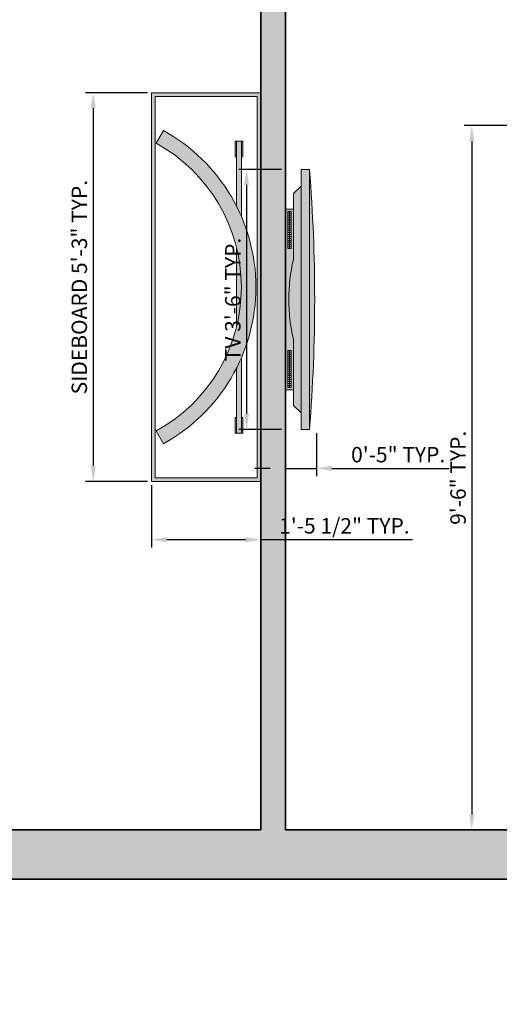
# Model space of a CAD drawing. Units: inches. Extents: x 1566 to 2546, y 1087 to 2705.
# Tile 14 of 27: x 2237 to 2315, y 1189 to 1349. Entities that reach past the tile are written whole.
import ezdxf

# ---------------------------------------------------------------- set-up
doc = ezdxf.new("R2010")
doc.units = ezdxf.units.IN
for name, color, linetype, lineweight in [('A-ANNO-DIMS', 2, 'Continuous', 18), ('A-FURN', 8, 'Continuous', 18), ('A-WALL', 7, 'Continuous', 35), ('A-WALL-PATT', 8, 'Continuous', 13), ('aparador', 36, 'Continuous', 9), ('moveis', 254, 'Continuous', 5), ('parede', 7, 'Continuous', 30)]:
    doc.layers.add(name, color=color, linetype=linetype, lineweight=lineweight)
doc.styles.get("Standard").update_dxf_attribs({"font": 'arial.ttf'})
doc.dimstyles.new('ISO-25', dxfattribs={"dimtxt": 2.5, "dimasz": 2.5, "dimexe": 1.25, "dimexo": 0.625, "dimtad": 1, "dimtxsty": 'Standard', "dimcen": 2.5, "dimadec": 0, "dimazin": 0, "dimtfac": 1, "dimtmove": 0, "dimatfit": 3, "dimfxl": 1, "dimarcsym": 0})

# ---------------------------------------------------------------- blocks, each defined once
blk = doc.blocks.new('Aparador ORGANICA Formatto')
at = {"layer": 'aparador', "ltscale": 0.3}
h = blk.add_hatch(color=256, dxfattribs=at)
h.dxf.hatch_style = 1
h.set_gradient(color1=(118, 213, 123), color2=(52, 168, 57), one_color=1, tint=0.43, name='INVCURVED')
h.paths.add_polyline_path([(0.8, 0.45), (-0.8, 0.45), (-0.8, 0), (0.8, 0)])
h.paths.add_polyline_path([(0.785, 0.435), (0.785, 0.015), (-0.785, 0.015), (-0.785, 0.435)], flags=16)
h.paths.add_polyline_path([(0.2911, 0.3699), (0.5365, 0.3699), (0.5365, 0.3757), (0.6011, 0.3757), (0.6011, 0.3699), (0.6011, 0.3499), (0.6011, 0.3441), (0.5365, 0.3441), (0.5365, 0.3499), (0.3338, 0.3499, -0.150336), (0.6449, 0.0488), (0.5923, 0.0199, 0.208852), (0.1632, 0.3499), (-0.1632, 0.3499, 0.208852), (-0.5923, 0.0199), (-0.6449, 0.0488, -0.150336), (-0.3338, 0.3499), (-0.5365, 0.3499), (-0.5365, 0.3441), (-0.6011, 0.3441), (-0.6011, 0.3499), (-0.6011, 0.3699), (-0.6011, 0.3757), (-0.5365, 0.3757), (-0.5365, 0.3699), (-0.2911, 0.3699, -0.206106)], flags=0)
h = blk.add_hatch(color=256, dxfattribs=at)
h.dxf.hatch_style = 1
h.set_gradient(color1=(135, 92, 69), color2=(0, 0, 0), one_color=1, name='INVCURVED')
h.paths.add_polyline_path([(-0.6449, 0.0488), (-0.5923, 0.0199, -0.590888), (0.5923, 0.0199), (0.6449, 0.0488, 0.590888)])
h = blk.add_hatch(color=256, dxfattribs=at)
h.dxf.hatch_style = 1
h.set_gradient(color1=(178, 189, 189), one_color=1, tint=1, name='CYLINDER')
h.paths.add_polyline_path([(-0.5365, 0.3757), (-0.6011, 0.3757), (-0.6011, 0.3699), (-0.5365, 0.3699)])
h.paths.add_polyline_path([(-0.5365, 0.3499), (-0.6011, 0.3499), (-0.6011, 0.3441), (-0.5365, 0.3441)])
h = blk.add_hatch(color=256, dxfattribs=at)
h.dxf.hatch_style = 1
h.set_gradient(color1=(118, 213, 123), color2=(31, 101, 35), one_color=1, tint=0.26, name='INVCURVED')
h.paths.add_polyline_path([(-0.2911, 0.3699), (-0.6011, 0.3699), (-0.6011, 0.3499), (-0.3338, 0.3499, -0.015999)])
h = blk.add_hatch(color=256, dxfattribs=at)
h.dxf.hatch_style = 1
h.set_gradient(color1=(118, 213, 123), color2=(31, 101, 35), one_color=1, tint=0.26, name='INVCURVED')
h.paths.add_polyline_path([(-0.1632, 0.3499), (0.1632, 0.3499, 0.122516)])
h = blk.add_hatch(color=256, dxfattribs=at)
h.dxf.hatch_style = 1
h.set_gradient(color1=(118, 213, 123), color2=(31, 101, 35), one_color=1, tint=0.26, name='INVCURVED')
h.paths.add_polyline_path([(0.6011, 0.3699), (0.2911, 0.3699, -0.015999), (0.3338, 0.3499), (0.6011, 0.3499)])
h = blk.add_hatch(color=256, dxfattribs=at)
h.dxf.hatch_style = 1
h.set_gradient(color1=(178, 189, 189), one_color=1, tint=1, name='CYLINDER')
h.paths.add_polyline_path([(0.6011, 0.3757), (0.5365, 0.3757), (0.5365, 0.3699), (0.6011, 0.3699)])
h.paths.add_polyline_path([(0.6011, 0.3499), (0.5365, 0.3499), (0.5365, 0.3441), (0.6011, 0.3441)])
for p, q in [((-0.5923, 0.0199), (-0.6449, 0.0488)), ((0.5923, 0.0199), (0.6449, 0.0488))]:
    blk.add_line(p, q, dxfattribs=at)
for points in [[(-0.6011, 0.3699), (-0.6011, 0.3757), (-0.5365, 0.3757), (-0.5365, 0.3699)], [(0.6011, 0.3699), (0.6011, 0.3757), (0.5365, 0.3757), (0.5365, 0.3699)], [(-0.5365, 0.3499), (-0.5365, 0.3441), (-0.6011, 0.3441), (-0.6011, 0.3499)], [(0.5365, 0.3499), (0.5365, 0.3441), (0.6011, 0.3441), (0.6011, 0.3499)]]:
    blk.add_lwpolyline(points, dxfattribs=at)
for radius in [0.7362, 0.6762]:
    blk.add_arc((0, -0.3063), radius, 28.8434, 151.1566, dxfattribs=at)
at = {"layer": 'moveis', "ltscale": 0.3}
for p, q in [((-0.6011, 0.3699), (-0.6011, 0.3499)), ((-0.2911, 0.3699), (-0.6011, 0.3699)), ((0.2911, 0.3699), (0.6011, 0.3699)), ((0.6011, 0.3699), (0.6011, 0.3499)), ((-0.6011, 0.3499), (-0.3338, 0.3499)), ((-0.1632, 0.3499), (0.1632, 0.3499)), ((0.6011, 0.3499), (0.3338, 0.3499))]:
    blk.add_line(p, q, dxfattribs=at)
for points in [[(-0.8, 0), (0.8, 0), (0.8, 0.45), (-0.8, 0.45)], [(-0.785, 0.015), (0.785, 0.015), (0.785, 0.435), (-0.785, 0.435)]]:
    blk.add_lwpolyline(points, close=True, dxfattribs=at)
blk = doc.blocks.new('PLASMA 2')
at = {"layer": 'moveis', "ltscale": 0.08}
h = blk.add_hatch(dxfattribs=at)
h.set_pattern_fill('_USER,_O', color=256, scale=0.008, double=1, pattern_type=0)
h.set_pattern_definition([(360, (-4.134502, -6.848382), (0, 0.008), []), (90, (-4.134502, -6.848382), (-0.008, 0), [])])
h.paths.add_polyline_path([(-0.2099, -0.0965), (-0.3623, -0.0965), (-0.3623, -0.1111), (-0.2099, -0.1111)])
h = blk.add_hatch(dxfattribs=at)
h.set_pattern_fill('_USER,_O', color=256, scale=0.008, double=1, pattern_type=0)
h.set_pattern_definition([(180, (4.134502, -6.848382), (0, 0.008), []), (90, (4.134502, -6.848382), (0.008, 0), [])])
h.paths.add_polyline_path([(0.2099, -0.0965), (0.3623, -0.0965), (0.3623, -0.1111), (0.2099, -0.1111)])
at = {"layer": 'parede', "ltscale": 0.08}
h = blk.add_hatch(color=256, dxfattribs=at)
h.dxf.hatch_style = 1
h.set_gradient(color1=(131, 136, 145), one_color=1, tint=1, name='CURVED')
h.paths.add_polyline_path([(-0.535, -0.0215), (0.535, -0.0215, 0.040195)])
h = blk.add_hatch(color=256, dxfattribs=at)
h.dxf.hatch_style = 1
h.set_gradient(color1=(131, 136, 145), color2=(0, 0, 0), one_color=1, name='CURVED')
h.paths.add_polyline_path([(0.535, -0.0215), (-0.535, -0.0215), (-0.535, -0.0553), (0.535, -0.0553)])
h = blk.add_hatch(color=256, dxfattribs=at)
h.dxf.hatch_style = 1
h.set_gradient(color1=(131, 136, 145), one_color=1, tint=1, name='CYLINDER')
h.paths.add_polyline_path([(0.4673, -0.0553), (-0.4673, -0.0553), (-0.4363, -0.0876), (-0.1636, -0.0876, 0.114423), (0.1636, -0.0876), (0.4363, -0.0876)])
h = blk.add_hatch(color=256, dxfattribs=at)
h.dxf.hatch_style = 1
h.set_gradient(color1=(131, 136, 145), color2=(0, 0, 0), one_color=1, name='CURVED')
h.paths.add_polyline_path([(0.3724, -0.0876), (0.1636, -0.0876, -0.114423), (-0.1636, -0.0876), (-0.3724, -0.0876), (-0.3724, -0.12), (0.3724, -0.12)])
h.paths.add_polyline_path([(-0.2099, -0.1111), (-0.3623, -0.1111), (-0.3623, -0.0965), (-0.2099, -0.0965)], flags=16)
h.paths.add_polyline_path([(0.2099, -0.1111), (0.2099, -0.0965), (0.3623, -0.0965), (0.3623, -0.1111)], flags=16)
at = {"layer": 'moveis', "ltscale": 0.08}
for p, q in [((-0.535, -0.0215), (-0.535, -0.0553)), ((-0.535, -0.0215), (0.535, -0.0215)), ((0.535, -0.0553), (0.535, -0.0215)), ((0.535, -0.0553), (-0.535, -0.0553)), ((-0.4673, -0.0553), (-0.4363, -0.0876)), ((0.4673, -0.0553), (0.4363, -0.0876)), ((-0.4363, -0.0876), (-0.1636, -0.0876)), ((-0.3724, -0.0876), (-0.3724, -0.12)), ((-0.3724, -0.12), (0.3724, -0.12)), ((0.1636, -0.0876), (0.4363, -0.0876)), ((0.3724, -0.0876), (0.3724, -0.12))]:
    blk.add_line(p, q, dxfattribs=at)
for points in [[(-0.3623, -0.0965), (-0.2099, -0.0965), (-0.2099, -0.1111), (-0.3623, -0.1111)], [(0.3623, -0.0965), (0.2099, -0.0965), (0.2099, -0.1111), (0.3623, -0.1111)]]:
    blk.add_lwpolyline(points, close=True, dxfattribs=at)
for centre, radius, start, end in [((0, -6.6658), 6.6658, 85.39647, 94.60353), ((0, 0.6178), 0.7242, 256.9449, 283.0551)]:
    blk.add_arc(centre, radius, start, end, dxfattribs=at)
blk = doc.blocks.new('*D48')
at = {"layer": 'A-ANNO-DIMS', "color": 0, "lineweight": -2, "transparency": 16777216}
for p, q in [((2327.57, 1331.61), (2309.22, 1331.61)), ((2310.47, 1329.11), (2310.47, 1219.93)), ((2327.57, 1217.43), (2309.22, 1217.43))]:
    blk.add_line(p, q, dxfattribs=at)
at = {"layer": 'A-ANNO-DIMS', "color": 0, "transparency": 16777216}
for points in [[(2310.06, 1329.11), (2310.89, 1329.11), (2310.47, 1331.61)], [(2310.06, 1219.93), (2310.89, 1219.93), (2310.47, 1217.43)]]:
    blk.add_solid(points, dxfattribs=at)
at = {"layer": 'Defpoints', "color": 0, "transparency": 16777216}
for p in [(2328.19, 1331.61), (2310.47, 1217.43), (2328.19, 1217.43)]:
    blk.add_point(p, dxfattribs=at)
at = {"layer": 'A-ANNO-DIMS', "color": 0, "transparency": 16777216, "insert": (2308.57, 1274.52), "char_height": 2.5, "attachment_point": 5, "rotation": 90}
blk.add_mtext('9\'-6" TYP.', dxfattribs=at)
blk = doc.blocks.new('*D49')
at = {"layer": 'A-ANNO-DIMS', "color": 0, "lineweight": -2, "transparency": 16777216}
for p, q in [((2279.66, 1324.5), (2272.72, 1324.5)), ((2273.97, 1322), (2273.97, 1284.87)), ((2279.66, 1282.37), (2272.72, 1282.37))]:
    blk.add_line(p, q, dxfattribs=at)
at = {"layer": 'A-ANNO-DIMS', "color": 0, "transparency": 16777216}
for points in [[(2273.55, 1322), (2274.39, 1322), (2273.97, 1324.5)], [(2273.55, 1284.87), (2274.39, 1284.87), (2273.97, 1282.37)]]:
    blk.add_solid(points, dxfattribs=at)
at = {"layer": 'Defpoints', "color": 0, "transparency": 16777216}
for p in [(2280.29, 1324.5), (2273.97, 1282.37), (2280.29, 1282.37)]:
    blk.add_point(p, dxfattribs=at)
at = {"layer": 'A-ANNO-DIMS', "color": 0, "transparency": 16777216, "insert": (2272.07, 1303.43), "char_height": 2.5, "attachment_point": 5, "rotation": 90}
blk.add_mtext('TV 3\'-6" TYP.', dxfattribs=at)
blk = doc.blocks.new('*D50')
at = {"layer": 'A-ANNO-DIMS', "color": 0, "lineweight": -2, "transparency": 16777216}
for p, q in [((2280.29, 1281.74), (2280.29, 1274.8)), ((2285.3, 1281.74), (2285.3, 1274.8)), ((2277.79, 1276.05), (2275.29, 1276.05)), ((2280.29, 1276.05), (2285.3, 1276.05)), ((2287.8, 1276.05), (2306.78, 1276.05))]:
    blk.add_line(p, q, dxfattribs=at)
at = {"layer": 'A-ANNO-DIMS', "color": 0, "transparency": 16777216}
for points in [[(2277.79, 1276.47), (2277.79, 1275.63), (2280.29, 1276.05)], [(2287.8, 1276.47), (2287.8, 1275.63), (2285.3, 1276.05)]]:
    blk.add_solid(points, dxfattribs=at)
at = {"layer": 'Defpoints', "color": 0, "transparency": 16777216}
for p in [(2280.29, 1282.37), (2285.3, 1282.37), (2285.3, 1276.05)]:
    blk.add_point(p, dxfattribs=at)
at = {"layer": 'A-ANNO-DIMS', "color": 0, "transparency": 16777216, "insert": (2298.54, 1277.95), "char_height": 2.5, "attachment_point": 5}
blk.add_mtext('0\'-5" TYP.', dxfattribs=at)
blk = doc.blocks.new('*D57')
at = {"layer": 'A-ANNO-DIMS', "color": 0, "lineweight": -2, "transparency": 16777216}
for p, q in [((2257.95, 1336.93), (2247.87, 1336.93)), ((2249.12, 1334.43), (2249.12, 1276.44)), ((2257.95, 1273.94), (2247.87, 1273.94))]:
    blk.add_line(p, q, dxfattribs=at)
at = {"layer": 'A-ANNO-DIMS', "color": 0, "transparency": 16777216}
for points in [[(2248.71, 1334.43), (2249.54, 1334.43), (2249.12, 1336.93)], [(2248.71, 1276.44), (2249.54, 1276.44), (2249.12, 1273.94)]]:
    blk.add_solid(points, dxfattribs=at)
at = {"layer": 'Defpoints', "color": 0, "transparency": 16777216}
for p in [(2258.57, 1336.93), (2249.12, 1273.94), (2258.57, 1273.94)]:
    blk.add_point(p, dxfattribs=at)
at = {"layer": 'A-ANNO-DIMS', "color": 0, "transparency": 16777216, "insert": (2247.2, 1305.43), "char_height": 2.5, "attachment_point": 5, "rotation": 90}
blk.add_mtext('SIDEBOARD 5\'-3" TYP.', dxfattribs=at)
blk = doc.blocks.new('*D58')
at = {"layer": 'A-ANNO-DIMS', "color": 0, "lineweight": -2, "transparency": 16777216}
for p, q in [((2258.57, 1273.31), (2258.57, 1263.24)), ((2276.29, 1273.31), (2276.29, 1263.24)), ((2261.07, 1264.49), (2273.79, 1264.49)), ((2276.29, 1264.49), (2300.87, 1264.49))]:
    blk.add_line(p, q, dxfattribs=at)
at = {"layer": 'A-ANNO-DIMS', "color": 0, "transparency": 16777216}
for points in [[(2261.07, 1264.9), (2261.07, 1264.07), (2258.57, 1264.49)], [(2273.79, 1264.9), (2273.79, 1264.07), (2276.29, 1264.49)]]:
    blk.add_solid(points, dxfattribs=at)
at = {"layer": 'Defpoints', "color": 0, "transparency": 16777216}
for p in [(2258.57, 1273.94), (2276.29, 1273.94), (2276.29, 1264.49)]:
    blk.add_point(p, dxfattribs=at)
at = {"layer": 'A-ANNO-DIMS', "color": 0, "transparency": 16777216, "insert": (2289.83, 1266.41), "char_height": 2.5, "attachment_point": 5}
blk.add_mtext('1\'-5 1/2" TYP.', dxfattribs=at)

msp = doc.modelspace()

# ---------------------------------------------------------------- hatches: boundary and pattern name
at = {"layer": 'A-WALL-PATT'}
h = msp.add_hatch(color=256, dxfattribs=at)
h.dxf.hatch_style = 1
h.paths.add_polyline_path([(2106.29, 1385.43), (2228.29, 1385.43), (2228.29, 1391.43), (2224.29, 1391.43), (2224.29, 1389.43), (2106.29, 1389.43), (2106.29, 1402.93), (2098.29, 1402.93), (2098.29, 1343.43), (2106.29, 1343.43), (2106.29, 1347.74)], flags=17)
h.paths.add_polyline_path([(2106.29, 1259.43), (2098.29, 1259.43), (2098.29, 1209.43), (2155.29, 1209.43), (2155.29, 1217.43), (2143.41, 1217.43), (2106.29, 1217.43)], flags=17)
h.paths.add_polyline_path([(2334.29, 1217.43), (2280.29, 1217.43), (2280.29, 1389.43), (2284.29, 1389.43), (2284.29, 1391.43), (2284.29, 1393.43), (2276.29, 1393.43), (2276.29, 1217.43), (2227.29, 1217.43), (2227.29, 1209.43), (2334.29, 1209.43)], flags=17)
h.paths.add_polyline_path([(2106.29, 1486.43), (2098.29, 1486.43), (2098.29, 1460.88), (2099.11, 1461.64), (2100.44, 1462.65), (2101.57, 1463.26), (2099.97, 1460.62), (2098.29, 1458.1), (2098.29, 1456.93), (2100.35, 1456.93), (2100.77, 1457.12), (2103.56, 1457.95), (2106.29, 1458.4), (2106.29, 1470.43), (2224.29, 1470.43), (2224.29, 1427.43), (2228.29, 1427.43), (2228.29, 1474.43), (2192.29, 1474.43), (2192.29, 1476.43), (2188.29, 1476.43), (2188.29, 1474.43), (2106.29, 1474.43)], flags=17)
h.paths.add_polyline_path([(2106.29, 1585.43), (2192.29, 1585.43), (2192.29, 1589.43), (2098.29, 1589.43), (2098.29, 1573.93), (2106.29, 1573.93)], flags=17)
h.paths.add_polyline_path([(2228.29, 1585.43), (2232.29, 1585.43), (2232.29, 1589.43), (2224.29, 1589.43), (2222.29, 1589.43), (2222.29, 1585.43), (2224.29, 1585.43), (2224.29, 1532.43), (2106.29, 1532.43), (2106.29, 1543.93), (2098.29, 1543.93), (2098.29, 1516.43), (2106.29, 1516.43), (2106.29, 1528.43), (2188.29, 1528.43), (2188.29, 1506.43), (2192.29, 1506.43), (2192.29, 1528.43), (2224.29, 1528.43), (2224.29, 1506.43), (2228.29, 1506.43)], flags=17)
h.paths.add_polyline_path([(2106.29, 1680.43), (2098.29, 1680.43), (2098.29, 1625.43), (2106.29, 1625.43)], flags=17)
h.paths.add_polyline_path([(2458.29, 1784.43), (2098.29, 1784.43), (2098.29, 1776.43), (2276.29, 1776.43), (2276.29, 1589.43), (2268.29, 1589.43), (2268.29, 1585.43), (2280.29, 1585.43), (2280.29, 1652.43), (2284.29, 1652.43), (2284.29, 1656.43), (2280.29, 1656.43), (2280.29, 1776.43), (2398.29, 1776.43), (2398.29, 1746.43), (2402.29, 1746.43), (2402.29, 1776.43), (2450.29, 1776.43), (2450.29, 1532.43), (2375.49, 1532.43), (2328.29, 1532.43), (2328.29, 1612.43), (2324.29, 1612.43), (2324.29, 1528.43), (2450.29, 1528.43), (2450.29, 1447.43), (2291.29, 1447.43), (2291.29, 1443.43), (2324.29, 1443.43), (2324.29, 1393.43), (2320.29, 1393.43), (2320.29, 1389.43), (2330.29, 1389.43), (2330.29, 1393.43), (2328.29, 1393.43), (2328.29, 1443.43), (2412.29, 1443.43), (2412.29, 1433.43), (2416.29, 1433.43), (2416.29, 1443.43), (2450.29, 1443.43), (2450.29, 1393.43), (2416.29, 1393.43), (2416.29, 1403.43), (2412.29, 1403.43), (2412.29, 1393.43), (2360.29, 1393.43), (2360.29, 1389.43), (2450.29, 1389.43), (2450.29, 1217.43), (2396.29, 1217.43), (2396.29, 1209.43), (2450.29, 1209.43), (2450.29, 1136.43), (2458.29, 1136.43)])

# ---------------------------------------------------------------- linework, layer by layer
at = {"layer": 'A-WALL'}
for p, q in [((2276.29, 1217.43), (2276.29, 1393.43)), ((2280.29, 1217.43), (2280.29, 1389.43)), ((2106.29, 1217.43), (2276.29, 1217.43)), ((2280.29, 1217.43), (2450.29, 1217.43)), ((2098.29, 1209.43), (2450.29, 1209.43))]:
    msp.add_line(p, q, dxfattribs=at)

# ---------------------------------------------------------------- block references
at = {"layer": 'A-FURN', "xscale": 39.3701, "yscale": 39.3701, "zscale": 39.3701, "rotation": 270}
for name, p in [('Aparador ORGANICA Formatto', (2258.57, 1305.43)), ('PLASMA 2', (2285.01, 1303.43))]:
    msp.add_blockref(name, p, dxfattribs=at)

# ---------------------------------------------------------------- dimensions: what is measured, and where the dimension line sits
at = {"layer": 'A-ANNO-DIMS'}
for base, p1, p2, text, picture, middle in [((2249.12, 1273.94), (2258.57, 1336.93), (2258.57, 1273.94), 'SIDEBOARD <> TYP.', '*D57', (2247.2, 1305.43)), ((2310.47, 1217.43), (2328.19, 1331.61), (2328.19, 1217.43), '<> TYP.', '*D48', (2308.57, 1274.52)), ((2273.97, 1282.37), (2280.29, 1324.5), (2280.29, 1282.37), 'TV <> TYP.', '*D49', (2272.07, 1303.43))]:
    dim = msp.add_linear_dim(base=base, p1=p1, p2=p2, angle=270, text=text, dimstyle='ISO-25', override={"dimdec": 1, "dimrnd": 0, "dimzin": 1, "dimlunit": 4, "dimfrac": 2}, dxfattribs=at)
    dim.commit()
    dim.dimension.update_dxf_attribs({"geometry": picture, "text_midpoint": middle})
for base, p1, p2, picture, middle in [((2285.3, 1276.05), (2280.29, 1282.37), (2285.3, 1282.37), '*D50', (2298.54, 1277.95)), ((2276.29, 1264.49), (2258.57, 1273.94), (2276.29, 1273.94), '*D58', (2289.83, 1266.41))]:
    dim = msp.add_linear_dim(base=base, p1=p1, p2=p2, text='<> TYP.', dimstyle='ISO-25', override={"dimdec": 1, "dimrnd": 0, "dimzin": 1, "dimlunit": 4, "dimfrac": 2}, dxfattribs=at)
    dim.commit()
    dim.dimension.update_dxf_attribs({"geometry": picture, "text_midpoint": middle})

doc.saveas('drawing.dxf')
